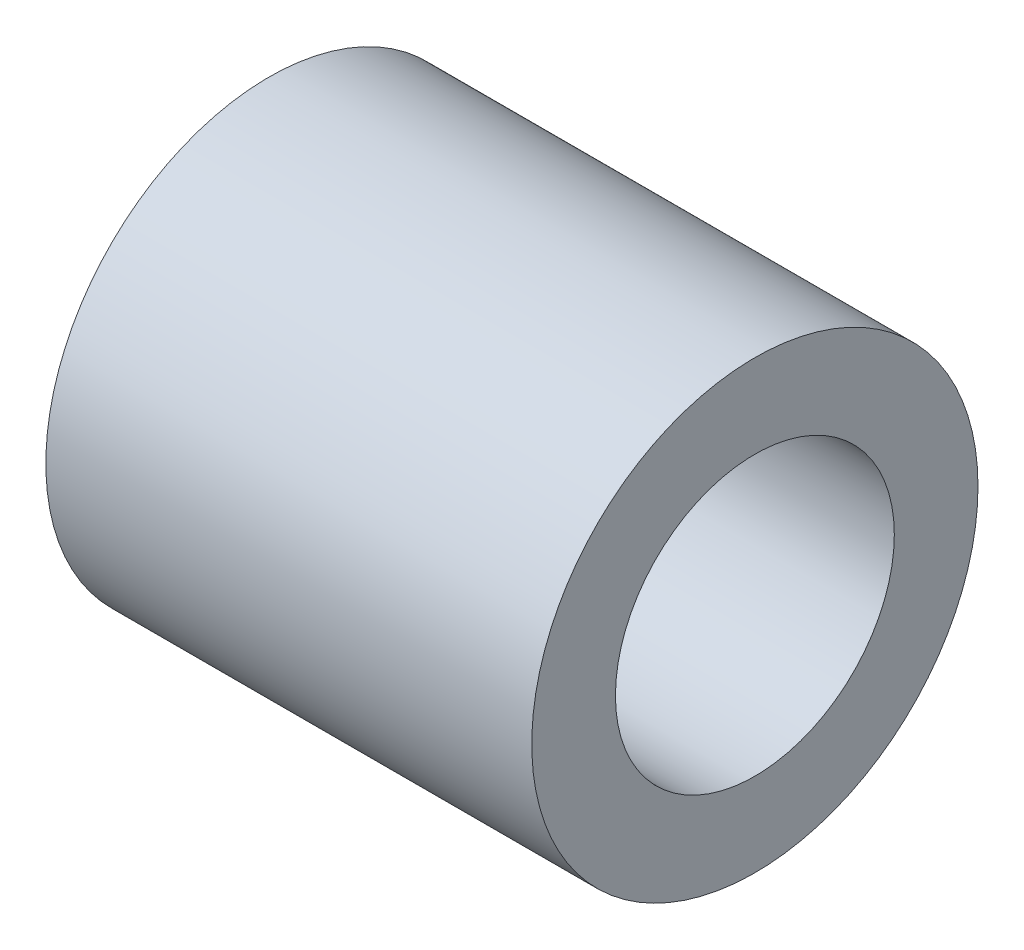
SolidWorks part; units mm, degrees
material "Plain Carbon Steel"
ref_plane "Front Plane" through (0, 0, 0) normal (0, 0, 1) x (1, 0, 0)
ref_plane "Top Plane" through (0, 0, 0) normal (0, 1, 0) x (1, 0, 0)
ref_plane "Right Plane" through (0, 0, 0) normal (1, 0, 0) x (0, 0, -1)
sketch "Cap Body Sketch Ø8" plane through (0, 0, 0) normal (1, 0, 0) x (0, 0, -1)
  line L0 (-112.1276, 0) -> (5494.2508, 0) construction
  line L1 (0, -112.1276) -> (0, 5494.2508) construction
  circle A0 centre (0, 0) radius 4
  dimension "D1" = 8
extrude "Cap Body Ø8x9" add sketch "Cap Body Sketch Ø8" along normal blind 9
sketch "Bore Drill Point Sketch" plane through (0, 0, 0) normal (0, 0, 1) x (1, 0, 0)
  line L0 (-1000, 0) -> (49000, 0) construction
  line L1 (0, 4) -> (0, -4) construction
  line L2 (0, 3.5) -> (0.7002, 4.7128)
  line L3 (0.7002, 4.7128) -> (0, 4.7128)
  line L4 (0, 4.7128) -> (0, 3.5)
  dimension "D1" = 3.5
  dimension "D2" = 1.2128
  dimension "D3" = 0.7002
revolve "Bore Drill Point Cut" cut sketch "Bore Drill Point Sketch" angle 360 about L0
sketch "Bore Sketch Ø5" plane through (9, 0, 0) normal (1, 0, 0) x (0, 0, -1)
  circle A0 centre (0, 0) radius 2.5
  dimension "D1" = 5
extrude "Bore Ø5x6" cut sketch "Bore Sketch Ø5" against normal blind 6
